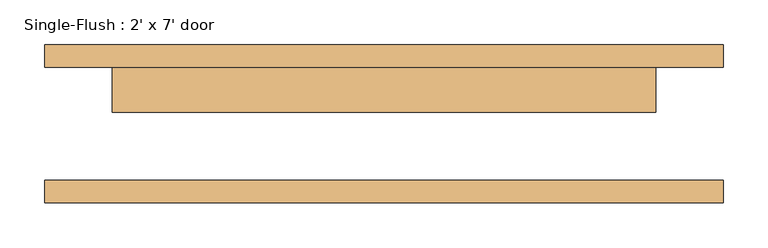
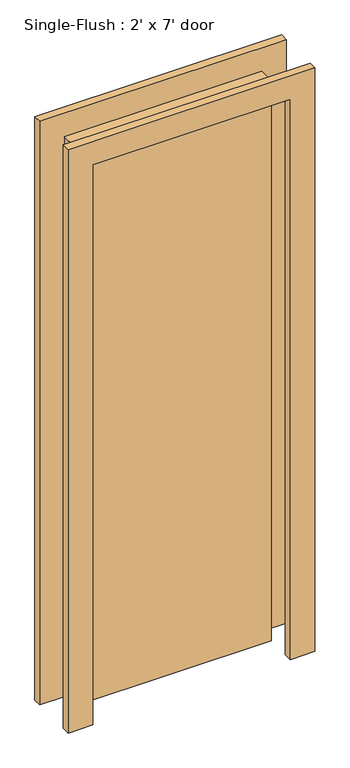
"""IFC4 building model written with IfcOpenShell, lengths in millimetres: door geometry, Single-Flush : 2' x 7' door."""

from ifc_helpers import new_model, si_unit, frame, origin, origin_with_axes, place, context, project, spatial, polyline, outline, extrude, source, transform, mapped, element, save


def single_flush_2_x_7_door_01f1079d(model_context):
    return source(origin(), model_context, "Body", "SweptSolid", [
        extrude(outline(polyline([(1905.0, -381.0), (0.0, -381.0), (0.0, -304.8), (1828.8, -304.8), (1828.8, 304.8), (0.0, 304.8), (0.0, 381.0), (1905.0, 381.0), (1905.0, -381.0)])), frame((0.0, 63.5, 0.0), z_axis=(0.0, 1.0, 0.0), x_axis=(0.0, 0.0, 1.0)), (0.0, 0.0, 1.0), 25.4),
        extrude(outline(polyline([(1905.0, 381.0), (1905.0, -381.0), (0.0, -381.0), (0.0, -304.8), (1828.8, -304.8), (1828.8, 304.8), (0.0, 304.8), (0.0, 381.0), (1905.0, 381.0)])), frame((0.0, -88.9, 0.0), z_axis=(0.0, 1.0, 0.0), x_axis=(0.0, 0.0, 1.0)), (0.0, 0.0, 1.0), 25.4),
        extrude(outline(polyline([(304.8, 12.7), (-304.8, 12.7), (-304.8, 63.5), (304.8, 63.5), (304.8, 12.7)])), origin_with_axes(), (0.0, 0.0, 1.0), 1828.8),
    ])


if __name__ == "__main__":
    model = new_model("IFC4")
    model_context = context("Model", 3, world=origin())
    ifc_project = project(units=[si_unit("LENGTHUNIT", "METRE", prefix="MILLI")], contexts=[model_context])
    site = spatial("IfcSite", under=ifc_project)
    building = spatial("IfcBuilding", under=site)
    placement = place(None, origin())
    single_flush_2_x_7_door_shape = single_flush_2_x_7_door_01f1079d(model_context)
    element("IfcDoor", 1, ObjectType="Single-Flush : 2' x 7' door", at=placement, inside=building, context=model_context, shape_type="MappedRepresentation", body=[
        mapped(single_flush_2_x_7_door_shape, transform((0.0, 0.0, 0.0), x_axis=(1.0, 0.0, 0.0), y_axis=(0.0, 1.0, 0.0), z_axis=(0.0, 0.0, 1.0))),
    ])
    save(model, "model.ifc")

# Revit data of these elements
# Type "Single-Flush : 2' x 7' door"
#   Type Mark = "18"
#   Construction Type Id = "MDOOR"
#   Assembly Code = "C1020"
#   Analytic Construction = "Metal"
#   Thickness = 0' - 2"
#   Heat Transfer Coefficient (U) = 0.651978 BTU/(h·ft²·°F)
#   Height = 6' - 0"
#   Trim Projection Ext = 0' - 1"
#   Trim Projection Int = 0' - 1"
#   Trim Width = 0' - 3"
#   Width = 2' - 0"
#   Define Thermal Properties by = 1
#   Door Material = Door - Panel
#   Frame Material = Door - Frame
#   Visual Light Transmittance = 0
#   Solar Heat Gain Coefficient = 0
#   Function = (empty or 0)
#   Wall Closure = (empty or 0)
# Element 1 (IfcDoor, "Single-Flush : 2' x 7' door")
#   Materials on its faces: "Door - Frame", "Door - Panel"
# Materials
#   "Door - Panel": class "Wood", colour RGB 210 159 95, transparency 0, Cost = 0
#   "Door - Frame": colour RGB 118 70 51, transparency 0, Cost = 0
